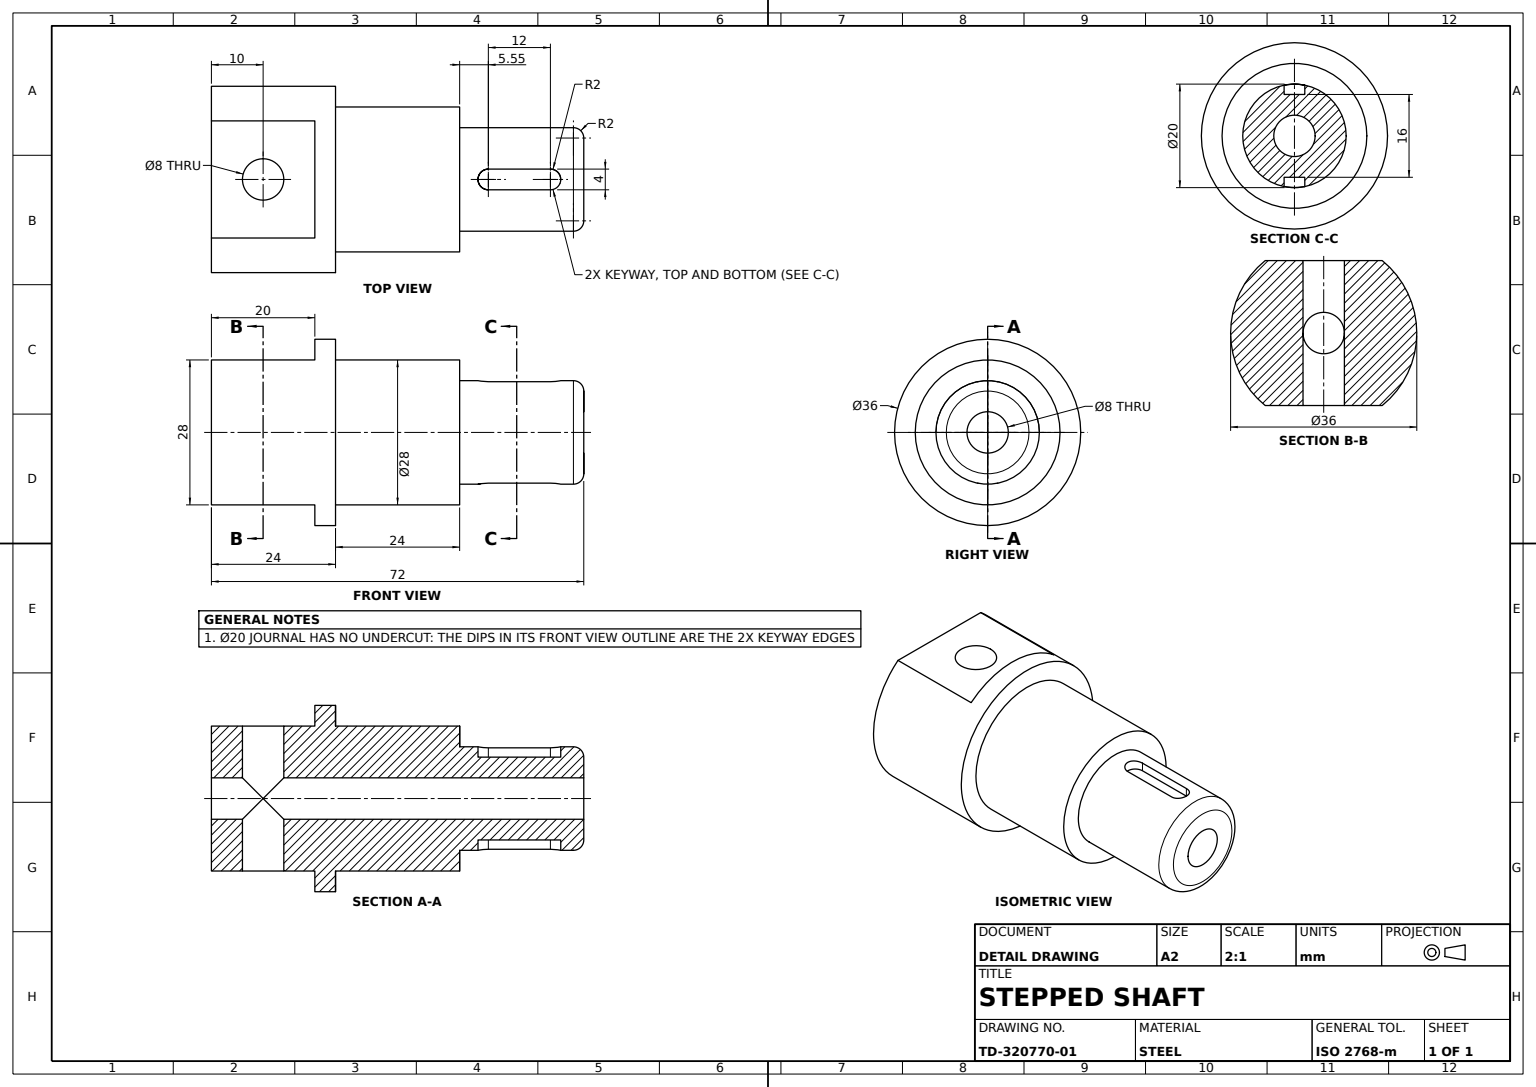
from build123d import *

# Parameters (mm, degrees)
BASE_START          = -20
BASE_FLAT_DEPTH     = 20
CROSS_HOLE_SKETCH_R = 4
CROSS_HOLE_8_DEPTH  = 30
EDGE_FILLET_R2_R    = 2
SLOT_2X16_DEPTH     = 2


with BuildPart() as part:
    # Shaft Profile Sketch → Stepped Shaft Body (revolve)
    with BuildSketch(Plane.XY, mode=Mode.PRIVATE) as stepped_shaft_body_sk:
        Polygon((4, 72), (4, 0), (18, 0), (18, 24), (14, 24), (14, 48), (10, 48), (10, 72), align=None)
    revolve(stepped_shaft_body_sk.sketch.rotate(Axis((0, -40.631578947, 0), (0, 1, 0)), 90), axis=Axis((0, -40.631578947, 0), (0, 1, 0)))

    # Base Flat Sketch → Base Flat (cut)
    with BuildSketch(Plane.XZ.offset(BASE_START)):
        with BuildLine():
            Line((-14, 11.313708499), (-14, -11.313708499))
            ThreePointArc((-14, -11.313708499), (-18, 0), (-14, 11.313708499))
        make_face()
        with BuildLine():
            Line((14, 11.313708499), (14, -11.313708499))
            ThreePointArc((14, -11.313708499), (18, 0), (14, 11.313708499))
        make_face()
    extrude(amount=BASE_FLAT_DEPTH, mode=Mode.SUBTRACT)

    # Cross Hole Sketch → Cross Hole Ø8 (cut)
    with BuildSketch(Plane.ZY.offset(14)):
        with Locations((0, 10)):
            Circle(CROSS_HOLE_SKETCH_R)
    extrude(amount=-CROSS_HOLE_8_DEPTH, mode=Mode.SUBTRACT)

    # Edge Fillet R2
    edge_fillet_r2_edges = [part.edges().sort_by_distance(p)[0] for p in [
        (0, 72, 10),
    ]]
    fillet(edge_fillet_r2_edges, radius=EDGE_FILLET_R2_R)

    # Slot Sketch → Slot 2x16 (cut)
    with BuildSketch(Plane(origin=(8, 0, 0), x_dir=(0, 0, -1), z_dir=(1, 0, 0))):
        with BuildLine():
            Line((2, 65.548124709), (2, 53.548124709))
            ThreePointArc((2, 53.548124709), (0, 51.548124709), (-2, 53.548124709))
            Line((-2, 53.548124709), (-2, 65.548124709))
            ThreePointArc((-2, 65.548124709), (0, 67.548124709), (2, 65.548124709))
        make_face()
    slot_2x16 = extrude(amount=SLOT_2X16_DEPTH, mode=Mode.SUBTRACT)

    # Slot Mirror: Slot 2x16 across plane
    add(slot_2x16.mirror(Plane(origin=(0, 0, 0), x_dir=(0, 0, 1), z_dir=(1, 0, 0))), mode=Mode.SUBTRACT)


solid = part.part
